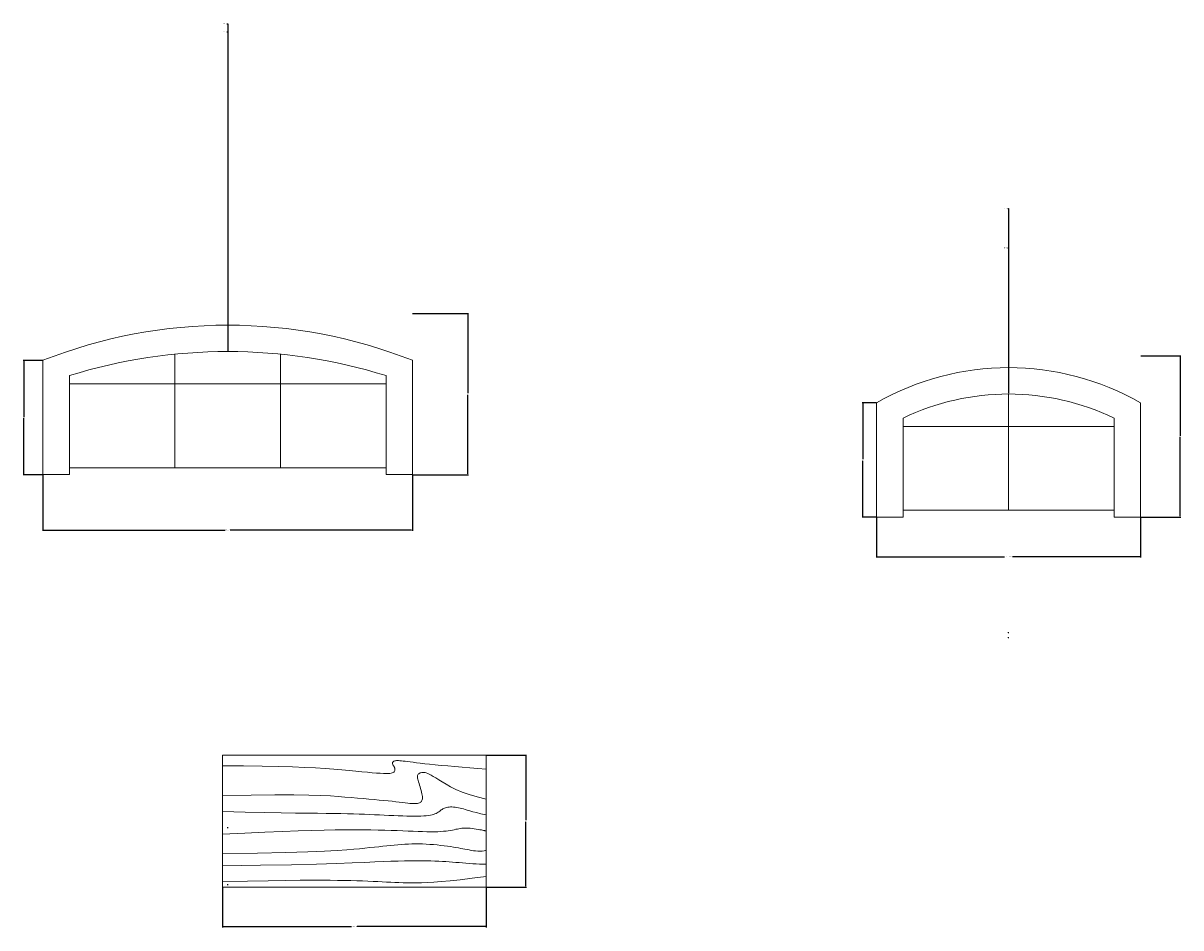
# Model space of a CAD drawing. Units: inches. Extents: x -52 to 1967, y 32 to 824.
# Tile 7 of 10: x 1540 to 1803, y 83 to 289. Entities that reach past the tile are written whole.
import ezdxf

# ---------------------------------------------------------------- set-up
doc = ezdxf.new("R2010")
doc.units = ezdxf.units.IN
doc.layers.add('A-ANNO-DIMS', color=2, linetype='Continuous', lineweight=18)
doc.layers.add('A-FURN', color=8, linetype='Continuous', lineweight=18)
doc.styles.get("Standard").update_dxf_attribs({"font": 'arial.ttf'})
doc.dimstyles.get("Standard").update_dxf_attribs({"dimtxt": 0.18, "dimasz": 0.18, "dimexe": 0.18, "dimexo": 0.0625, "dimgap": 0.09, "dimtad": 0, "dimtih": 1, "dimtoh": 1, "dimdec": 4, "dimzin": 0, "dimdsep": 46, "dimtxsty": 'Standard', "dimcen": 0.09, "dimadec": 0, "dimazin": 0, "dimtfac": 1, "dimtdec": 4, "dimtofl": 0, "dimtmove": 0, "dimatfit": 3, "dimfxl": 1, "dimtolj": 1, "dimtzin": 0, "dimarcsym": 0})

# ---------------------------------------------------------------- blocks, each defined once
blk = doc.blocks.new('Sofa - Roundback 7 ft.')
for p, q in [((-12.00002, -32.4421), (-12.00003, -6.5971)), ((11.99997, -32.4421), (11.99998, -6.5971)), ((-36.000027, -34), (-36.000027, -11.4696)), ((35.99998, -34), (35.99998, -11.4696)), ((-35.999844, -13.3819), (35.9998, -13.3819)), ((-36.000027, -32.4421), (35.99998, -32.4421))]:
    blk.add_line(p, q)
for points in [[(-36.000027, -34), (-42.000027, -34), (-42.000027, -8)], [(41.99998, -8), (41.99998, -34), (35.99998, -34)]]:
    blk.add_lwpolyline(points)
for centre, radius, start, end in [((0, -114.25), 114.25, 68.43141, 111.5686), ((-0.00001, -127.1968), 121.1968, 72.72033, 107.2797)]:
    blk.add_arc(centre, radius, start, end)
blk = doc.blocks.new('Sofa - Roundback Loveseat 5 ft.')
for p, q in [((0, -32.44198), (0, -5.99998)), ((-24, -33.99998), (-24, -11.46958)), ((24.00004, -33.99998), (24.00004, -11.46958)), ((-23.9998, -13.38178), (23.99986, -13.38178)), ((-24, -32.44198), (24.00004, -32.44198))]:
    blk.add_line(p, q)
for points in [[(-24, -33.99998), (-30, -33.99998), (-30, -7.99998)], [(30.00004, -7.99998), (30.00004, -33.99998), (24.00004, -33.99998)]]:
    blk.add_lwpolyline(points)
for centre, radius, start, end in [((0, -60.24998), 60.24998, 60.13715, 119.8628), ((0, -61.38438), 55.38444, 64.32083, 115.6792)]:
    blk.add_arc(centre, radius, start, end)
blk = doc.blocks.new('Table - Rectangular Woodgrain 60 x 30 in.')
for p, q in [((0, 0), (0, -30)), ((60, 0), (0, 0)), ((60, -30), (60, 0)), ((0, -30), (60, -30))]:
    blk.add_line(p, q)
for points in [[(0, -2.4), (4.8155, -2.418), (9.0302, -2.4688), (12.709, -2.5477), (15.9167, -2.65), (18.7181, -2.7711), (21.1781, -2.9063), (23.3616, -3.0508), (25.3333, -3.2), (27.1477, -3.3495), (28.8172, -3.4958), (30.3437, -3.636), (31.7291, -3.7667), (32.9756, -3.8849), (34.0849, -3.9875), (35.059, -4.0714), (35.9, -4.1334), (36.6114, -4.1711), (37.2041, -4.1854), (37.6906, -4.1779), (38.0833, -4.15), (38.3948, -4.1034), (38.6375, -4.0396), (38.8239, -3.9602), (38.9666, -3.8667), (39.0764, -3.7608), (39.1573, -3.6448), (39.2116, -3.521), (39.2416, -3.3917), (39.2498, -3.2593), (39.2385, -3.1261), (39.21, -2.9944), (39.1666, -2.8667), (39.111, -2.7447), (39.0468, -2.6281), (38.978, -2.5163), (38.9083, -2.4083), (38.8418, -2.3035), (38.7823, -2.201), (38.7337, -2.1001), (38.7, -2), (38.6844, -1.9003), (38.6875, -1.8021), (38.7094, -1.707), (38.75, -1.6167), (38.8094, -1.5326), (38.8875, -1.4563), (38.9844, -1.3893), (39.1, -1.3333), (39.2351, -1.2896), (39.3937, -1.2583), (39.5804, -1.2396), (39.8, -1.2333), (40.057, -1.2396), (40.3562, -1.2583), (40.7023, -1.2896), (41.1, -1.3333), (41.5547, -1.3895), (42.0755, -1.4573), (42.6721, -1.5361), (43.3542, -1.625), (44.1316, -1.7233), (45.014, -1.8302), (46.0114, -1.9449), (47.1333, -2.0667), (48.3862, -2.1947), (49.7625, -2.3281), (51.2513, -2.4663), (52.8416, -2.6083), (54.5226, -2.7535), (56.2833, -2.9011), (58.1127, -3.0501), (60, -3.2)], [(0, -9.2), (6.5759, -9.0858), (11.9385, -9.0365), (16.2527, -9.0418), (19.6833, -9.0917), (22.3952, -9.1759), (24.5531, -9.2844), (26.322, -9.4069), (27.8666, -9.5333), (29.3241, -9.6553), (30.7203, -9.7719), (32.0532, -9.8837), (33.3208, -9.9917), (34.5213, -10.0965), (35.6526, -10.199), (36.7128, -10.2999), (37.7, -10.4), (38.6129, -10.4996), (39.4531, -10.5969), (40.223, -10.6895), (40.925, -10.775), (41.5613, -10.8512), (42.1344, -10.9156), (42.6465, -10.966), (43.1, -11), (43.4976, -11.0158), (43.8437, -11.0136), (44.143, -10.9942), (44.4, -10.9583), (44.6195, -10.9069), (44.8062, -10.8406), (44.9648, -10.7603), (45.1, -10.6667), (45.2155, -10.5598), (45.3114, -10.4365), (45.3871, -10.2929), (45.4416, -10.125), (45.4743, -9.929), (45.4844, -9.7011), (45.4709, -9.4371), (45.4333, -9.1333), (45.3716, -8.7883), (45.2896, -8.4104), (45.1919, -8.0107), (45.0833, -7.6), (44.9685, -7.1893), (44.8521, -6.7896), (44.7388, -6.4117), (44.6333, -6.0667), (44.54, -5.7628), (44.4614, -5.4979), (44.4001, -5.2675), (44.3583, -5.0667), (44.3384, -4.8909), (44.3427, -4.7354), (44.3736, -4.5956), (44.4333, -4.4667), (44.5236, -4.3453), (44.6427, -4.2333), (44.7884, -4.1339), (44.9583, -4.05), (45.1501, -3.9849), (45.3614, -3.9417), (45.59, -3.9234), (45.8333, -3.9333), (46.0915, -3.9749), (46.3734, -4.0531), (46.6906, -4.1736), (47.0542, -4.3417), (47.4756, -4.5629), (47.9661, -4.8427), (48.5372, -5.1866), (49.2, -5.6), (49.9676, -6.0844), (50.8594, -6.625), (51.8965, -7.2031), (53.1, -7.8), (54.491, -8.3969), (56.0906, -8.975), (57.9199, -9.5156), (60, -10)], [(0, -12.8), (5.1847, -12.9322), (9.6213, -13.0323), (13.3963, -13.1059), (16.5958, -13.1583), (19.3063, -13.1952), (21.614, -13.2219), (23.6054, -13.2439), (25.3666, -13.2667), (26.9728, -13.2947), (28.4531, -13.3281), (29.8256, -13.3663), (31.1083, -13.4083), (32.3191, -13.4535), (33.476, -13.501), (34.597, -13.5501), (35.7, -13.6), (36.7984, -13.6497), (37.8875, -13.6979), (38.9578, -13.743), (40, -13.7833), (41.0047, -13.8174), (41.9625, -13.8438), (42.864, -13.8607), (43.7, -13.8667), (44.4631, -13.8604), (45.1552, -13.8417), (45.7801, -13.8104), (46.3416, -13.7667), (46.8439, -13.7104), (47.2906, -13.6417), (47.6858, -13.5604), (48.0333, -13.4667), (48.3375, -13.3608), (48.6042, -13.2448), (48.8396, -13.121), (49.05, -12.9917), (49.2417, -12.8593), (49.4208, -12.7261), (49.5937, -12.5944), (49.7667, -12.4667), (49.9452, -12.3451), (50.1323, -12.2313), (50.3303, -12.1268), (50.5416, -12.0333), (50.7686, -11.9524), (51.0135, -11.8854), (51.2788, -11.8341), (51.5666, -11.8), (51.8785, -11.7843), (52.2116, -11.7865), (52.562, -11.8059), (52.926, -11.8417), (53.2998, -11.8931), (53.6795, -11.9594), (54.0614, -12.0397), (54.4416, -12.1333), (54.8223, -12.2401), (55.2293, -12.3625), (55.6942, -12.5037), (56.2489, -12.6667), (56.9251, -12.8547), (57.7545, -13.0708), (58.7689, -13.3182), (60, -13.6)], [(0, -18), (5.124, -17.7273), (9.6609, -17.5057), (13.6705, -17.3303), (17.2125, -17.1958), (20.3467, -17.0973), (23.1328, -17.0297), (25.6307, -16.9878), (27.9, -16.9667), (29.9928, -16.9617), (31.9302, -16.9703), (33.7254, -16.9907), (35.3917, -17.0208), (36.9423, -17.0588), (38.3906, -17.1026), (39.7499, -17.1503), (41.0333, -17.2), (42.2519, -17.2496), (43.4073, -17.2969), (44.4986, -17.3395), (45.525, -17.375), (46.4858, -17.4012), (47.3802, -17.4156), (48.2074, -17.416), (48.9667, -17.4), (49.6583, -17.3662), (50.2872, -17.3167), (50.8595, -17.2547), (51.3812, -17.1833), (51.8584, -17.1057), (52.2971, -17.025), (52.7034, -16.9443), (53.0833, -16.8667), (53.443, -16.7951), (53.789, -16.7313), (54.128, -16.6768), (54.4666, -16.6334), (54.8115, -16.6024), (55.1693, -16.5854), (55.5465, -16.5841), (55.95, -16.6), (56.3828, -16.6337), (56.8346, -16.6823), (57.2915, -16.7418), (57.7396, -16.8084), (58.165, -16.878), (58.5539, -16.9469), (58.8924, -17.0111), (59.1666, -17.0667), (59.3679, -17.1107), (59.5078, -17.1438), (59.6032, -17.1675), (59.6708, -17.1833), (59.7275, -17.193), (59.7901, -17.1979), (59.8753, -17.1998), (60, -17.2)], [(0, -22.4), (8.0098, -22.2501), (14.4094, -22.1011), (19.4168, -21.9535), (23.25, -21.8083), (26.1269, -21.6663), (28.2656, -21.5281), (29.884, -21.3947), (31.2, -21.2667), (32.3967, -21.1448), (33.5172, -21.0292), (34.5697, -20.9198), (35.5625, -20.8167), (36.5037, -20.7198), (37.4015, -20.6292), (38.2642, -20.5448), (39.1, -20.4667), (39.9164, -20.3951), (40.7187, -20.3313), (41.5117, -20.2768), (42.3, -20.2333), (43.0883, -20.2024), (43.8812, -20.1854), (44.6836, -20.1841), (45.5, -20.2), (46.3328, -20.234), (47.1747, -20.2844), (48.0163, -20.3488), (48.8479, -20.425), (49.66, -20.5106), (50.4429, -20.6031), (51.1872, -20.7004), (51.8833, -20.8), (52.5246, -20.8999), (53.1166, -20.9995), (53.6681, -21.0983), (54.1875, -21.1958), (54.6834, -21.2919), (55.1646, -21.3859), (55.6394, -21.4777), (56.1167, -21.5667), (56.6028, -21.6515), (57.0961, -21.7266), (57.5929, -21.7852), (58.0896, -21.8208), (58.5823, -21.8268), (59.0674, -21.7964), (59.5412, -21.723), (60, -21.6)], [(0, -25.2), (8.6355, -25.0504), (15.7026, -24.9031), (21.4049, -24.7606), (25.9458, -24.625), (29.529, -24.4988), (32.3578, -24.3844), (34.6359, -24.284), (36.5667, -24.2), (38.3213, -24.1341), (39.9417, -24.0854), (41.437, -24.0523), (42.8167, -24.0333), (44.0901, -24.0268), (45.2667, -24.0313), (46.3557, -24.0451), (47.3667, -24.0667), (48.309, -24.0947), (49.1928, -24.1287), (50.0284, -24.168), (50.826, -24.2125), (51.5959, -24.2617), (52.3483, -24.3151), (53.0935, -24.3725), (53.8417, -24.4334), (54.6009, -24.497), (55.3699, -24.561), (56.1454, -24.6226), (56.9239, -24.6792), (57.7021, -24.7279), (58.4764, -24.7662), (59.2435, -24.7911), (60, -24.8)], [(0, -28.8), (5.6867, -28.6681), (10.45, -28.5698), (14.407, -28.5012), (17.675, -28.4584), (20.3711, -28.4374), (22.6125, -28.4344), (24.5164, -28.4455), (26.2, -28.4667), (27.762, -28.4947), (29.2276, -28.5281), (30.6033, -28.5663), (31.8958, -28.6084), (33.1118, -28.6535), (34.2578, -28.7011), (35.3405, -28.7501), (36.3666, -28.8), (37.3443, -28.8497), (38.288, -28.8974), (39.2137, -28.9412), (40.1375, -28.9792), (41.0753, -29.0093), (42.0432, -29.0297), (43.0572, -29.0384), (44.1333, -29.0333), (45.2936, -29.0114), (46.5843, -28.9641), (48.0579, -28.8816), (49.7666, -28.7542), (51.7629, -28.5721), (54.0989, -28.3255), (56.8272, -28.0048), (60, -27.6)]]:
    blk.add_lwpolyline(points)
blk = doc.blocks.new('*D33')
at = {"layer": 'A-ANNO-DIMS', "color": 0, "lineweight": -2, "transparency": 16777216}
for p, q in [((1544.28, 185.9), (1544.28, 173.18)), ((1628.28, 185.9), (1628.28, 173.18)), ((1544.46, 173.36), (1585.68, 173.36)), ((1628.1, 173.36), (1586.87, 173.36))]:
    blk.add_line(p, q, dxfattribs=at)
at = {"layer": 'A-ANNO-DIMS', "color": 0, "transparency": 16777216}
for points in [[(1544.46, 173.39), (1544.46, 173.33), (1544.28, 173.36)], [(1628.1, 173.39), (1628.1, 173.33), (1628.28, 173.36)]]:
    blk.add_solid(points, dxfattribs=at)
at = {"layer": 'Defpoints', "color": 0, "transparency": 16777216}
for p in [(1544.28, 185.96), (1628.28, 185.96), (1628.28, 173.36)]:
    blk.add_point(p, dxfattribs=at)
at = {"layer": 'A-ANNO-DIMS', "color": 0, "transparency": 16777216, "insert": (1586.28, 173.36), "char_height": 0.18, "attachment_point": 5}
blk.add_mtext('\\A1;SOFA 84', dxfattribs=at)
blk = doc.blocks.new('*D34')
at = {"layer": 'A-ANNO-DIMS', "color": 0, "lineweight": -2, "transparency": 16777216}
for p, q in [((1628.34, 222.63), (1641.06, 222.63)), ((1640.88, 222.45), (1640.88, 204.48)), ((1640.88, 186.14), (1640.88, 204.12)), ((1628.34, 185.96), (1641.06, 185.96))]:
    blk.add_line(p, q, dxfattribs=at)
at = {"layer": 'A-ANNO-DIMS', "color": 0, "transparency": 16777216}
for points in [[(1640.85, 222.45), (1640.91, 222.45), (1640.88, 222.63)], [(1640.85, 186.14), (1640.91, 186.14), (1640.88, 185.96)]]:
    blk.add_solid(points, dxfattribs=at)
at = {"layer": 'Defpoints', "color": 0, "transparency": 16777216}
for p in [(1628.28, 222.63), (1640.88, 222.63), (1628.28, 185.96)]:
    blk.add_point(p, dxfattribs=at)
at = {"layer": 'A-ANNO-DIMS', "color": 0, "transparency": 16777216, "insert": (1640.88, 204.3), "char_height": 0.18, "attachment_point": 5}
blk.add_mtext('\\A1;37', dxfattribs=at)
blk = doc.blocks.new('*D35')
at = {"layer": 'A-ANNO-DIMS', "color": 0, "lineweight": -2, "transparency": 16777216}
for p, q in [((1733.84, 176.25), (1733.84, 167.13)), ((1793.84, 176.25), (1793.84, 167.13)), ((1734.02, 167.31), (1762.93, 167.31)), ((1793.66, 167.31), (1764.76, 167.31))]:
    blk.add_line(p, q, dxfattribs=at)
at = {"layer": 'A-ANNO-DIMS', "color": 0, "transparency": 16777216}
for points in [[(1734.02, 167.34), (1734.02, 167.28), (1733.84, 167.31)], [(1793.66, 167.34), (1793.66, 167.28), (1793.84, 167.31)]]:
    blk.add_solid(points, dxfattribs=at)
at = {"layer": 'Defpoints', "color": 0, "transparency": 16777216}
for p in [(1733.84, 176.31), (1793.84, 176.31), (1793.84, 167.31)]:
    blk.add_point(p, dxfattribs=at)
at = {"layer": 'A-ANNO-DIMS', "color": 0, "transparency": 16777216, "insert": (1763.84, 167.31), "char_height": 0.18, "attachment_point": 5}
blk.add_mtext('\\A1;LOVESEAT 60', dxfattribs=at)
blk = doc.blocks.new('*D36')
at = {"layer": 'A-ANNO-DIMS', "color": 0, "lineweight": -2, "transparency": 16777216}
for p, q in [((1793.9, 212.97), (1803.02, 212.97)), ((1802.84, 212.79), (1802.84, 194.82)), ((1802.84, 176.49), (1802.84, 194.46)), ((1793.9, 176.31), (1803.02, 176.31))]:
    blk.add_line(p, q, dxfattribs=at)
at = {"layer": 'A-ANNO-DIMS', "color": 0, "transparency": 16777216}
for points in [[(1802.81, 212.79), (1802.87, 212.79), (1802.84, 212.97)], [(1802.81, 176.49), (1802.87, 176.49), (1802.84, 176.31)]]:
    blk.add_solid(points, dxfattribs=at)
at = {"layer": 'Defpoints', "color": 0, "transparency": 16777216}
for p in [(1793.84, 212.97), (1802.84, 212.97), (1793.84, 176.31)]:
    blk.add_point(p, dxfattribs=at)
at = {"layer": 'A-ANNO-DIMS', "color": 0, "transparency": 16777216, "insert": (1802.84, 194.64), "char_height": 0.18, "attachment_point": 5}
blk.add_mtext('\\A1;37', dxfattribs=at)
blk = doc.blocks.new('*D39')
at = {"layer": 'A-ANNO-DIMS', "color": 0, "lineweight": -2, "transparency": 16777216}
for p, q in [((1585.07, 92.12), (1585.07, 83.01)), ((1645.07, 92.12), (1645.07, 83.01)), ((1585.25, 83.19), (1614.42, 83.19)), ((1644.89, 83.19), (1615.72, 83.19))]:
    blk.add_line(p, q, dxfattribs=at)
at = {"layer": 'A-ANNO-DIMS', "color": 0, "transparency": 16777216}
for points in [[(1585.25, 83.22), (1585.25, 83.16), (1585.07, 83.19)], [(1644.89, 83.22), (1644.89, 83.16), (1645.07, 83.19)]]:
    blk.add_solid(points, dxfattribs=at)
at = {"layer": 'Defpoints', "color": 0, "transparency": 16777216}
for p in [(1585.07, 92.19), (1645.07, 92.19), (1645.07, 83.19)]:
    blk.add_point(p, dxfattribs=at)
at = {"layer": 'A-ANNO-DIMS', "color": 0, "transparency": 16777216, "insert": (1615.07, 83.19), "char_height": 0.18, "attachment_point": 5}
blk.add_mtext('\\A1;TABLE 60', dxfattribs=at)
blk = doc.blocks.new('*D40')
at = {"layer": 'A-ANNO-DIMS', "color": 0, "lineweight": -2, "transparency": 16777216}
for p, q in [((1645.13, 122.19), (1654.25, 122.19)), ((1654.07, 122.01), (1654.07, 107.37)), ((1654.07, 92.37), (1654.07, 107)), ((1645.13, 92.19), (1654.25, 92.19))]:
    blk.add_line(p, q, dxfattribs=at)
at = {"layer": 'A-ANNO-DIMS', "color": 0, "transparency": 16777216}
for points in [[(1654.04, 122.01), (1654.1, 122.01), (1654.07, 122.19)], [(1654.04, 92.37), (1654.1, 92.37), (1654.07, 92.19)]]:
    blk.add_solid(points, dxfattribs=at)
at = {"layer": 'Defpoints', "color": 0, "transparency": 16777216}
for p in [(1645.07, 122.19), (1654.07, 122.19), (1645.07, 92.19)]:
    blk.add_point(p, dxfattribs=at)
at = {"layer": 'A-ANNO-DIMS', "color": 0, "transparency": 16777216, "insert": (1654.07, 107.19), "char_height": 0.18, "attachment_point": 5}
blk.add_mtext('\\A1;30', dxfattribs=at)
blk = doc.blocks.new('*D124')
at = {"layer": 'A-ANNO-DIMS', "color": 0, "lineweight": -2, "transparency": 16777216}
for p, q in [((1544.22, 211.96), (1539.77, 211.96)), ((1539.95, 211.78), (1539.95, 199.15)), ((1539.95, 186.14), (1539.95, 198.78)), ((1544.22, 185.96), (1539.77, 185.96))]:
    blk.add_line(p, q, dxfattribs=at)
at = {"layer": 'A-ANNO-DIMS', "color": 0, "transparency": 16777216}
for points in [[(1539.92, 211.78), (1539.98, 211.78), (1539.95, 211.96)], [(1539.92, 186.14), (1539.98, 186.14), (1539.95, 185.96)]]:
    blk.add_solid(points, dxfattribs=at)
at = {"layer": 'Defpoints', "color": 0, "transparency": 16777216}
for p in [(1539.95, 211.96), (1544.28, 211.96), (1544.28, 185.96)]:
    blk.add_point(p, dxfattribs=at)
at = {"layer": 'A-ANNO-DIMS', "color": 0, "transparency": 16777216, "insert": (1539.95, 198.96), "char_height": 0.18, "attachment_point": 5}
blk.add_mtext('\\A1;26', dxfattribs=at)
blk = doc.blocks.new('*D125')
at = {"layer": 'A-ANNO-DIMS', "color": 0, "lineweight": -2, "transparency": 16777216}
for p, q in [((1733.78, 202.31), (1730.53, 202.31)), ((1730.71, 202.13), (1730.71, 189.49)), ((1730.71, 176.49), (1730.71, 189.13)), ((1733.78, 176.31), (1730.53, 176.31))]:
    blk.add_line(p, q, dxfattribs=at)
at = {"layer": 'A-ANNO-DIMS', "color": 0, "transparency": 16777216}
for points in [[(1730.68, 202.13), (1730.74, 202.13), (1730.71, 202.31)], [(1730.68, 176.49), (1730.74, 176.49), (1730.71, 176.31)]]:
    blk.add_solid(points, dxfattribs=at)
at = {"layer": 'Defpoints', "color": 0, "transparency": 16777216}
for p in [(1730.71, 202.31), (1733.84, 202.31), (1733.84, 176.31)]:
    blk.add_point(p, dxfattribs=at)
at = {"layer": 'A-ANNO-DIMS', "color": 0, "transparency": 16777216, "insert": (1730.71, 189.31), "char_height": 0.18, "attachment_point": 5}
blk.add_mtext('\\A1;26', dxfattribs=at)
blk = doc.blocks.new('*D148')
at = {"layer": 'A-ANNO-DIMS', "color": 0, "lineweight": -2, "transparency": 16777216}
for p, q in [((1586.1, 288.51), (1586.28, 288.51)), ((1586.28, 288.51), (1586.28, 220.14)), ((1586.19, 105.71), (1586.37, 105.71)), ((1586.28, 105.62), (1586.28, 105.8))]:
    blk.add_line(p, q, dxfattribs=at)
at = {"layer": 'A-ANNO-DIMS', "color": 0, "transparency": 16777216}
blk.add_solid([(1586.31, 220.14), (1586.25, 220.14), (1586.28, 219.96)], dxfattribs=at)
at = {"layer": 'Defpoints', "color": 0, "transparency": 16777216}
for p in [(1586.28, 219.96), (1586.28, 105.71)]:
    blk.add_point(p, dxfattribs=at)
at = {"layer": 'A-ANNO-DIMS', "color": 0, "transparency": 16777216, "insert": (1585.55, 288.51), "char_height": 0.18, "attachment_point": 5}
blk.add_mtext('\\A1;R114.25', dxfattribs=at)
blk = doc.blocks.new('*D149')
at = {"layer": 'A-ANNO-DIMS', "color": 0, "lineweight": -2, "transparency": 16777216}
for p, q in [((1586.1, 286.68), (1586.28, 286.68)), ((1586.28, 286.68), (1586.28, 214.14)), ((1586.19, 92.77), (1586.37, 92.77)), ((1586.28, 92.68), (1586.28, 92.86))]:
    blk.add_line(p, q, dxfattribs=at)
at = {"layer": 'A-ANNO-DIMS', "color": 0, "transparency": 16777216}
blk.add_solid([(1586.31, 214.14), (1586.25, 214.14), (1586.28, 213.96)], dxfattribs=at)
at = {"layer": 'Defpoints', "color": 0, "transparency": 16777216}
for p in [(1586.28, 213.96), (1586.28, 92.77)]:
    blk.add_point(p, dxfattribs=at)
at = {"layer": 'A-ANNO-DIMS', "color": 0, "transparency": 16777216, "insert": (1585.62, 286.68), "char_height": 0.18, "attachment_point": 5}
blk.add_mtext('\\A1;R121.2', dxfattribs=at)
blk = doc.blocks.new('*D150')
at = {"layer": 'A-ANNO-DIMS', "color": 0, "lineweight": -2, "transparency": 16777216}
for p, q in [((1763.66, 246.46), (1763.84, 246.46)), ((1763.84, 246.46), (1763.84, 210.49)), ((1763.75, 150.06), (1763.93, 150.06)), ((1763.84, 149.97), (1763.84, 150.15))]:
    blk.add_line(p, q, dxfattribs=at)
at = {"layer": 'A-ANNO-DIMS', "color": 0, "transparency": 16777216}
blk.add_solid([(1763.87, 210.49), (1763.81, 210.49), (1763.84, 210.31)], dxfattribs=at)
at = {"layer": 'Defpoints', "color": 0, "transparency": 16777216}
for p in [(1763.84, 210.31), (1763.84, 150.06)]:
    blk.add_point(p, dxfattribs=at)
at = {"layer": 'A-ANNO-DIMS', "color": 0, "transparency": 16777216, "insert": (1763.18, 246.46), "char_height": 0.18, "attachment_point": 5}
blk.add_mtext('\\A1;R60.25', dxfattribs=at)
blk = doc.blocks.new('*D151')
at = {"layer": 'A-ANNO-DIMS', "color": 0, "lineweight": -2, "transparency": 16777216}
for p, q in [((1763.66, 237.54), (1763.84, 237.54)), ((1763.84, 237.54), (1763.84, 204.49)), ((1763.75, 148.92), (1763.93, 148.92)), ((1763.84, 148.83), (1763.84, 149.01))]:
    blk.add_line(p, q, dxfattribs=at)
at = {"layer": 'A-ANNO-DIMS', "color": 0, "transparency": 16777216}
blk.add_solid([(1763.87, 204.49), (1763.81, 204.49), (1763.84, 204.31)], dxfattribs=at)
at = {"layer": 'Defpoints', "color": 0, "transparency": 16777216}
for p in [(1763.84, 204.31), (1763.84, 148.92)]:
    blk.add_point(p, dxfattribs=at)
at = {"layer": 'A-ANNO-DIMS', "color": 0, "transparency": 16777216, "insert": (1763.18, 237.54), "char_height": 0.18, "attachment_point": 5}
blk.add_mtext('\\A1;R55.38', dxfattribs=at)

msp = doc.modelspace()

# ---------------------------------------------------------------- block references
at = {"layer": 'A-FURN'}
for name, p in [('Sofa - Roundback 7 ft.', (1586.2781, 219.9649)), ('Sofa - Roundback Loveseat 5 ft.', (1763.8418, 210.3077)), ('Table - Rectangular Woodgrain 60 x 30 in.', (1585.0702, 122.1852))]:
    msp.add_blockref(name, p, dxfattribs=at)

# ---------------------------------------------------------------- dimensions: what is measured, and where the dimension line sits
at = {"layer": 'A-ANNO-DIMS'}
for center, mpoint, override, picture, middle in [((1586.2781, 105.7149), (1586.278, 219.9649), {"dimdec": 2, "dimlfac": 1, "dimrnd": 0, "dimzin": 0, "dimdsep": 46, "dimlunit": 2}, '*D148', (1585.5475, 288.5149)), ((1586.2781, 92.7681), (1586.278, 213.9649), {"dimdec": 1, "dimlfac": 1, "dimrnd": 0, "dimzin": 0, "dimdsep": 46, "dimlunit": 2}, '*D149', (1585.619, 286.683)), ((1763.8418, 150.0577), (1763.84, 210.3077), {"dimdec": 2, "dimlfac": 1, "dimrnd": 0, "dimzin": 0, "dimdsep": 46, "dimlunit": 2}, '*D150', (1763.1784, 246.4576)), ((1763.8418, 148.9233), (1763.84, 204.3077), {"dimdec": 2, "dimlfac": 1, "dimrnd": 0, "dimzin": 0, "dimdsep": 46, "dimlunit": 2}, '*D151', (1763.1789, 237.5384))]:
    dim = msp.add_radius_dim(center=center, mpoint=mpoint, dimstyle='Standard', override=override, dxfattribs=at)
    dim.commit()
    dim.dimension.update_dxf_attribs({"geometry": picture, "text_midpoint": middle, "dimtype": 164})
for base, p1, p2, picture, middle in [((1640.8781, 222.6316), (1628.2781, 185.9649), (1628.2781, 222.6316), '*D34', (1640.8781, 204.2983)), ((1539.9481, 211.9649), (1544.2781, 185.9649), (1544.2781, 211.9649), '*D124', (1539.9481, 198.9649)), ((1802.8419, 212.9743), (1793.8419, 176.3077), (1793.8419, 212.9743), '*D36', (1802.8419, 194.641)), ((1730.7068, 202.3077), (1733.8418, 176.3077), (1733.8418, 202.3077), '*D125', (1730.7068, 189.3077)), ((1654.0702, 122.1852), (1645.0702, 92.1852), (1645.0702, 122.1852), '*D40', (1654.0702, 107.1852))]:
    dim = msp.add_linear_dim(base=base, p1=p1, p2=p2, angle=90, dimstyle='Standard', override={"dimdec": 0, "dimlfac": 1, "dimrnd": 0, "dimzin": 0, "dimdsep": 46, "dimlunit": 2}, dxfattribs=at)
    dim.commit()
    dim.dimension.update_dxf_attribs({"geometry": picture, "text_midpoint": middle})
for base, p1, p2, text, picture, middle in [((1628.2781, 173.3649), (1544.2781, 185.9649), (1628.2781, 185.9649), 'SOFA <>', '*D33', (1586.2781, 173.3649)), ((1793.8419, 167.3077), (1733.8418, 176.3077), (1793.8419, 176.3077), 'LOVESEAT <>', '*D35', (1763.8418, 167.3077)), ((1645.0702, 83.1852), (1585.0702, 92.1852), (1645.0702, 92.1852), 'TABLE <>', '*D39', (1615.0702, 83.1852))]:
    dim = msp.add_linear_dim(base=base, p1=p1, p2=p2, text=text, dimstyle='Standard', override={"dimdec": 0, "dimlfac": 1, "dimrnd": 0, "dimzin": 0, "dimdsep": 46, "dimlunit": 2}, dxfattribs=at)
    dim.commit()
    dim.dimension.update_dxf_attribs({"geometry": picture, "text_midpoint": middle})

doc.saveas('drawing.dxf')
